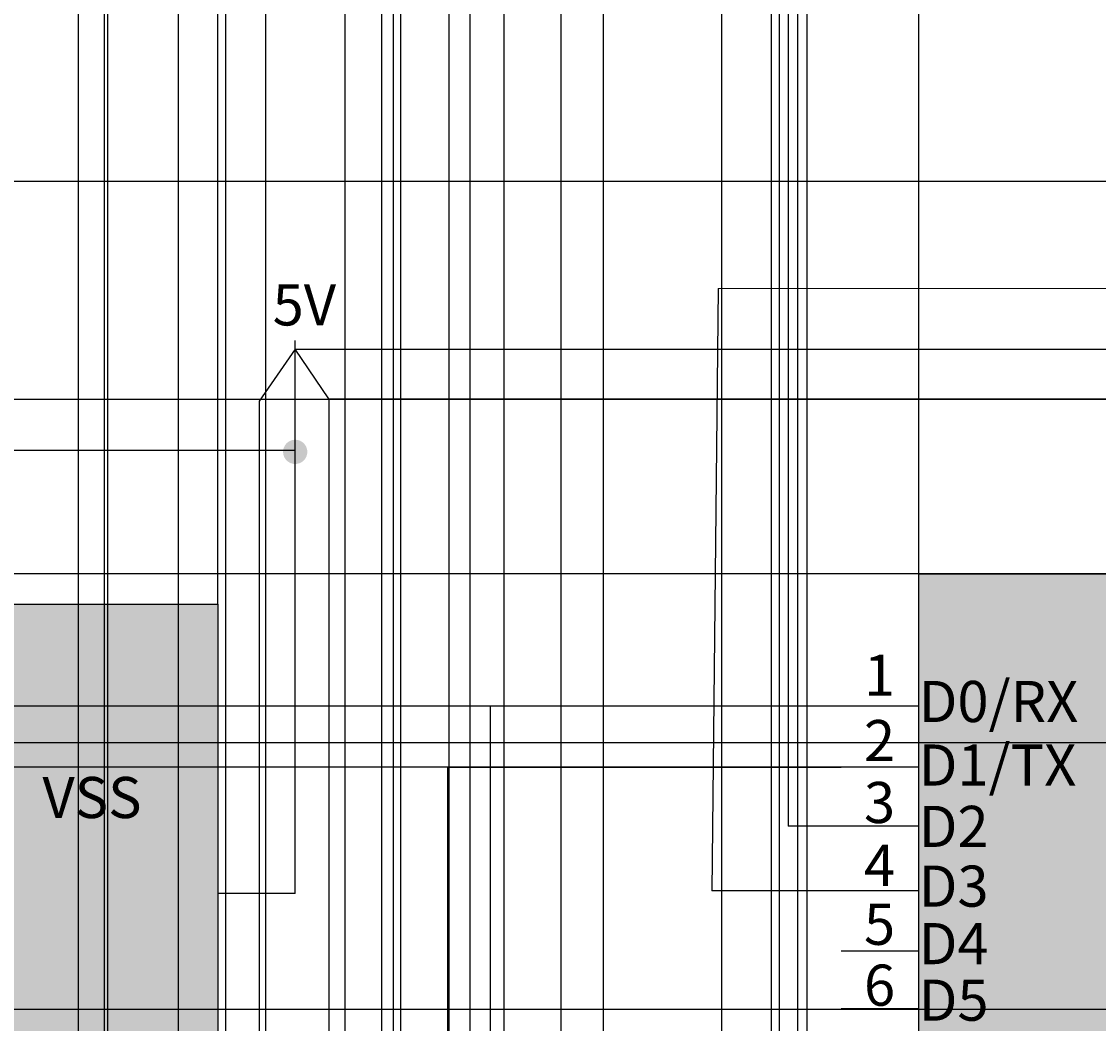
# Model space of a CAD drawing. Units: inches. Extents: x 35362 to 73946, y 43607 to 67532.
# Tile 131 of 134: x 52056 to 57838, y 56772 to 62152. Entities that reach past the tile are written whole.
import ezdxf

# ---------------------------------------------------------------- set-up
doc = ezdxf.new("R2010")
doc.units = ezdxf.units.IN
doc.header["$MEASUREMENT"] = 0
for name, color, linetype, lineweight in [('A-ANNO-DIMS', 2, 'Continuous', 18), ('E-ANNO-TEXT', 5, 'Continuous', 18), ('E-SYMB', 1, 'Continuous', 25), ('E-SYMB-PATT', 1, 'Continuous', 13), ('E-WIRE', 3, 'Continuous', 25)]:
    doc.layers.add(name, color=color, linetype=linetype, lineweight=lineweight)
doc.styles.get("Standard").update_dxf_attribs({"font": 'arial.ttf'})
doc.dimstyles.get("Standard").update_dxf_attribs({"dimtxt": 0.18, "dimasz": 0.18, "dimexe": 0.18, "dimexo": 0.0625, "dimgap": 0.09, "dimtad": 0, "dimtih": 1, "dimtoh": 1, "dimdec": 4, "dimzin": 0, "dimdsep": 46, "dimtxsty": 'Standard', "dimcen": 0.09, "dimadec": 0, "dimazin": 0, "dimtfac": 1, "dimtdec": 4, "dimtofl": 0, "dimtmove": 0, "dimatfit": 3, "dimfxl": 1, "dimtolj": 1, "dimtzin": 0, "dimarcsym": 0})

# ---------------------------------------------------------------- blocks, each defined once
blk = doc.blocks.new('*D9')
at = {"layer": 'A-ANNO-DIMS', "color": 0, "lineweight": -2, "transparency": 16777216}
for p, q in [((56873.6, 59185.2), (56873.6, 67531.7)), ((56873.8, 67531.5), (59056.9, 67531.5)), ((61240.7, 67531.5), (59057.6, 67531.5)), ((61240.9, 59185.2), (61240.9, 67531.7))]:
    blk.add_line(p, q, dxfattribs=at)
at = {"layer": 'A-ANNO-DIMS', "color": 0, "transparency": 16777216}
for points in [[(56873.8, 67531.5), (56873.8, 67531.5), (56873.6, 67531.5)], [(61240.7, 67531.5), (61240.7, 67531.5), (61240.9, 67531.5)]]:
    blk.add_solid(points, dxfattribs=at)
at = {"layer": 'Defpoints', "color": 0, "transparency": 16777216}
for p in [(61240.9, 67531.5), (56873.6, 59185.1), (61240.9, 59185.1)]:
    blk.add_point(p, dxfattribs=at)
at = {"layer": 'A-ANNO-DIMS', "color": 0, "transparency": 16777216, "insert": (59057.3, 67531.5), "char_height": 0.18, "attachment_point": 5}
blk.add_mtext('\\A1;4367', dxfattribs=at)
blk = doc.blocks.new('*D25')
at = {"layer": 'A-ANNO-DIMS', "color": 0, "lineweight": -2, "transparency": 16777216}
for p, q in [((53109.8, 59023.3), (53109.8, 67531.7)), ((53109.9, 67531.5), (54991.2, 67531.5)), ((56873.4, 67531.5), (54992.1, 67531.5)), ((56873.6, 59185.2), (56873.6, 67531.7))]:
    blk.add_line(p, q, dxfattribs=at)
at = {"layer": 'A-ANNO-DIMS', "color": 0, "transparency": 16777216}
for points in [[(53109.9, 67531.5), (53109.9, 67531.5), (53109.8, 67531.5)], [(56873.4, 67531.5), (56873.4, 67531.5), (56873.6, 67531.5)]]:
    blk.add_solid(points, dxfattribs=at)
at = {"layer": 'Defpoints', "color": 0, "transparency": 16777216}
for p in [(56873.6, 67531.5), (56873.6, 59185.1), (53109.8, 59023.3)]:
    blk.add_point(p, dxfattribs=at)
at = {"layer": 'A-ANNO-DIMS', "color": 0, "transparency": 16777216, "insert": (54991.7, 67531.5), "char_height": 0.18, "attachment_point": 5}
blk.add_mtext('\\A1;3763.8', dxfattribs=at)
blk = doc.blocks.new('*D34')
at = {"layer": 'A-ANNO-DIMS', "color": 0, "lineweight": -2, "transparency": 16777216}
for p, q in [((65336, 61293.3), (35361.8, 61293.3)), ((35361.9, 61293.1), (35361.9, 60239.4)), ((35361.9, 59185.3), (35361.9, 60239)), ((61240.8, 59185.1), (35361.8, 59185.1))]:
    blk.add_line(p, q, dxfattribs=at)
at = {"layer": 'A-ANNO-DIMS', "color": 0, "transparency": 16777216}
for points in [[(35361.9, 61293.1), (35362, 61293.1), (35361.9, 61293.3)], [(35361.9, 59185.3), (35362, 59185.3), (35361.9, 59185.1)]]:
    blk.add_solid(points, dxfattribs=at)
at = {"layer": 'Defpoints', "color": 0, "transparency": 16777216}
for p in [(65336, 61293.3), (35361.9, 59185.1), (61240.9, 59185.1)]:
    blk.add_point(p, dxfattribs=at)
at = {"layer": 'A-ANNO-DIMS', "color": 0, "transparency": 16777216, "insert": (35361.9, 60239.2), "char_height": 0.18, "attachment_point": 5}
blk.add_mtext('\\A1;2108.1', dxfattribs=at)
blk = doc.blocks.new('*D36')
at = {"layer": 'A-ANNO-DIMS', "color": 0, "lineweight": -2, "transparency": 16777216}
for p, q in [((68320.8, 60122.3), (35361.8, 60122.3)), ((35361.9, 60122.2), (35361.9, 57247.8)), ((35361.9, 54373.1), (35361.9, 57247.5)), ((68320.8, 54372.9), (35361.8, 54372.9))]:
    blk.add_line(p, q, dxfattribs=at)
at = {"layer": 'A-ANNO-DIMS', "color": 0, "transparency": 16777216}
for points in [[(35361.9, 60122.2), (35362, 60122.2), (35361.9, 60122.3)], [(35361.9, 54373.1), (35362, 54373.1), (35361.9, 54372.9)]]:
    blk.add_solid(points, dxfattribs=at)
at = {"layer": 'Defpoints', "color": 0, "transparency": 16777216}
for p in [(68320.9, 60122.3), (35361.9, 54372.9), (68320.9, 54372.9)]:
    blk.add_point(p, dxfattribs=at)
at = {"layer": 'A-ANNO-DIMS', "color": 0, "transparency": 16777216, "insert": (35361.9, 57247.6), "char_height": 0.18, "attachment_point": 5}
blk.add_mtext('\\A1;5749.4', dxfattribs=at)
blk = doc.blocks.new('*D39')
at = {"layer": 'A-ANNO-DIMS', "color": 0, "lineweight": -2, "transparency": 16777216}
for p, q in [((53793.6, 46128.9), (53793.6, 67531.7)), ((53793.8, 67531.5), (54487.2, 67531.5)), ((55181.5, 67531.5), (54488.1, 67531.5)), ((55181.6, 46128.9), (55181.6, 67531.7))]:
    blk.add_line(p, q, dxfattribs=at)
at = {"layer": 'A-ANNO-DIMS', "color": 0, "transparency": 16777216}
for points in [[(53793.8, 67531.5), (53793.8, 67531.5), (53793.6, 67531.5)], [(55181.5, 67531.5), (55181.5, 67531.5), (55181.6, 67531.5)]]:
    blk.add_solid(points, dxfattribs=at)
at = {"layer": 'Defpoints', "color": 0, "transparency": 16777216}
for p in [(55181.6, 67531.5), (53793.6, 46128.9), (55181.6, 46128.9)]:
    blk.add_point(p, dxfattribs=at)
at = {"layer": 'A-ANNO-DIMS', "color": 0, "transparency": 16777216, "insert": (54487.6, 67531.5), "char_height": 0.18, "attachment_point": 5}
blk.add_mtext('\\A1;1388.0', dxfattribs=at)
blk = doc.blocks.new('*D44')
at = {"layer": 'A-ANNO-DIMS', "color": 0, "lineweight": -2, "transparency": 16777216}
for p, q in [((52517.8, 64828.5), (52517.8, 43606.7)), ((54090.8, 64828.5), (54090.8, 43606.7)), ((52518, 43606.9), (53303.8, 43606.9)), ((54090.6, 43606.9), (53304.7, 43606.9))]:
    blk.add_line(p, q, dxfattribs=at)
at = {"layer": 'A-ANNO-DIMS', "color": 0, "transparency": 16777216}
for points in [[(52518, 43606.9), (52518, 43606.8), (52517.8, 43606.9)], [(54090.6, 43606.9), (54090.6, 43606.8), (54090.8, 43606.9)]]:
    blk.add_solid(points, dxfattribs=at)
at = {"layer": 'Defpoints', "color": 0, "transparency": 16777216}
for p in [(52517.8, 64828.6), (54090.8, 64828.6), (54090.8, 43606.9)]:
    blk.add_point(p, dxfattribs=at)
at = {"layer": 'A-ANNO-DIMS', "color": 0, "transparency": 16777216, "insert": (53304.3, 43606.9), "char_height": 0.18, "attachment_point": 5}
blk.add_mtext('\\A1;1573.0', dxfattribs=at)
blk = doc.blocks.new('*D47')
at = {"layer": 'A-ANNO-DIMS', "color": 0, "lineweight": -2, "transparency": 16777216}
for p, q in [((50339.6, 58280), (73945.8, 58280)), ((73945.6, 58279.8), (73945.6, 57564.2)), ((73945.6, 56848.2), (73945.6, 57563.8)), ((50339.6, 56848), (73945.8, 56848))]:
    blk.add_line(p, q, dxfattribs=at)
at = {"layer": 'A-ANNO-DIMS', "color": 0, "transparency": 16777216}
for points in [[(73945.6, 58279.8), (73945.7, 58279.8), (73945.6, 58280)], [(73945.6, 56848.2), (73945.7, 56848.2), (73945.6, 56848)]]:
    blk.add_solid(points, dxfattribs=at)
at = {"layer": 'Defpoints', "color": 0, "transparency": 16777216}
for p in [(50339.5, 58280), (50339.5, 56848), (73945.6, 56848)]:
    blk.add_point(p, dxfattribs=at)
at = {"layer": 'A-ANNO-DIMS', "color": 0, "transparency": 16777216, "insert": (73945.6, 57564), "char_height": 0.18, "attachment_point": 5}
blk.add_mtext('\\A1;1432.0', dxfattribs=at)
blk = doc.blocks.new('*D48')
at = {"layer": 'A-ANNO-DIMS', "color": 0, "lineweight": -2, "transparency": 16777216}
for p, q in [((56457.2, 58474.9), (35361.8, 58474.9)), ((35361.9, 58474.7), (35361.9, 58311.1)), ((35361.9, 58147.1), (35361.9, 58310.7)), ((56457.2, 58147), (35361.8, 58147))]:
    blk.add_line(p, q, dxfattribs=at)
at = {"layer": 'A-ANNO-DIMS', "color": 0, "transparency": 16777216}
for points in [[(35361.9, 58474.7), (35362, 58474.7), (35361.9, 58474.9)], [(35361.9, 58147.1), (35362, 58147.1), (35361.9, 58147)]]:
    blk.add_solid(points, dxfattribs=at)
at = {"layer": 'Defpoints', "color": 0, "transparency": 16777216}
for p in [(56457.3, 58474.9), (35361.9, 58147), (56457.3, 58147)]:
    blk.add_point(p, dxfattribs=at)
at = {"layer": 'A-ANNO-DIMS', "color": 0, "transparency": 16777216, "insert": (35361.9, 58310.9), "char_height": 0.18, "attachment_point": 5}
blk.add_mtext('\\A1;327.9', dxfattribs=at)
blk = doc.blocks.new('*D51')
at = {"layer": 'A-ANNO-DIMS', "color": 0, "lineweight": -2, "transparency": 16777216}
for p, q in [((56873.6, 59185.2), (56873.6, 67531.7)), ((56873.8, 67531.5), (57886, 67531.5)), ((58899.2, 67531.5), (57887, 67531.5)), ((58899.4, 59601.5), (58899.4, 67531.7))]:
    blk.add_line(p, q, dxfattribs=at)
at = {"layer": 'A-ANNO-DIMS', "color": 0, "transparency": 16777216}
for points in [[(56873.8, 67531.5), (56873.8, 67531.5), (56873.6, 67531.5)], [(58899.2, 67531.5), (58899.2, 67531.5), (58899.4, 67531.5)]]:
    blk.add_solid(points, dxfattribs=at)
at = {"layer": 'Defpoints', "color": 0, "transparency": 16777216}
for p in [(58899.4, 67531.5), (58899.4, 59601.5), (56873.6, 59185.1)]:
    blk.add_point(p, dxfattribs=at)
at = {"layer": 'A-ANNO-DIMS', "color": 0, "transparency": 16777216, "insert": (57886.5, 67531.5), "char_height": 0.18, "attachment_point": 5}
blk.add_mtext('\\A1;2025.8', dxfattribs=at)
blk = doc.blocks.new('*D77')
at = {"layer": 'A-ANNO-DIMS', "color": 0, "lineweight": -2, "transparency": 16777216}
for p, q in [((53793.6, 46128.9), (53793.6, 67531.7)), ((53793.8, 67531.5), (53922.8, 67531.5)), ((54052.7, 67531.5), (53923.7, 67531.5)), ((54052.9, 46555.4), (54052.9, 67531.7))]:
    blk.add_line(p, q, dxfattribs=at)
at = {"layer": 'A-ANNO-DIMS', "color": 0, "transparency": 16777216}
for points in [[(53793.8, 67531.5), (53793.8, 67531.5), (53793.6, 67531.5)], [(54052.7, 67531.5), (54052.7, 67531.5), (54052.9, 67531.5)]]:
    blk.add_solid(points, dxfattribs=at)
at = {"layer": 'Defpoints', "color": 0, "transparency": 16777216}
for p in [(54052.9, 67531.5), (54052.9, 46555.3), (53793.6, 46128.9)]:
    blk.add_point(p, dxfattribs=at)
at = {"layer": 'A-ANNO-DIMS', "color": 0, "transparency": 16777216, "insert": (53923.3, 67531.5), "char_height": 0.18, "attachment_point": 5}
blk.add_mtext('\\A1;259.26', dxfattribs=at)
blk = doc.blocks.new('*D78')
at = {"layer": 'A-ANNO-DIMS', "color": 0, "lineweight": -2, "transparency": 16777216}
for p, q in [((54052.9, 46555.4), (54052.9, 67531.7)), ((54053.1, 67531.5), (54202.6, 67531.5)), ((54352.9, 67531.5), (54203.4, 67531.5)), ((54353.1, 46555.4), (54353.1, 67531.7))]:
    blk.add_line(p, q, dxfattribs=at)
at = {"layer": 'A-ANNO-DIMS', "color": 0, "transparency": 16777216}
for points in [[(54053.1, 67531.5), (54053.1, 67531.5), (54052.9, 67531.5)], [(54352.9, 67531.5), (54352.9, 67531.5), (54353.1, 67531.5)]]:
    blk.add_solid(points, dxfattribs=at)
at = {"layer": 'Defpoints', "color": 0, "transparency": 16777216}
for p in [(54353.1, 67531.5), (54052.9, 46555.3), (54353.1, 46555.3)]:
    blk.add_point(p, dxfattribs=at)
at = {"layer": 'A-ANNO-DIMS', "color": 0, "transparency": 16777216, "insert": (54203, 67531.5), "char_height": 0.18, "attachment_point": 5}
blk.add_mtext('\\A1;300.2', dxfattribs=at)
blk = doc.blocks.new('*D79')
at = {"layer": 'A-ANNO-DIMS', "color": 0, "lineweight": -2, "transparency": 16777216}
for p, q in [((54353.1, 46555.4), (54353.1, 67531.7)), ((54353.3, 67531.5), (54500.2, 67531.5)), ((54648, 67531.5), (54501, 67531.5)), ((54648.2, 46555.4), (54648.2, 67531.7))]:
    blk.add_line(p, q, dxfattribs=at)
at = {"layer": 'A-ANNO-DIMS', "color": 0, "transparency": 16777216}
for points in [[(54353.3, 67531.5), (54353.3, 67531.5), (54353.1, 67531.5)], [(54648, 67531.5), (54648, 67531.5), (54648.2, 67531.5)]]:
    blk.add_solid(points, dxfattribs=at)
at = {"layer": 'Defpoints', "color": 0, "transparency": 16777216}
for p in [(54648.2, 67531.5), (54353.1, 46555.3), (54648.2, 46555.3)]:
    blk.add_point(p, dxfattribs=at)
at = {"layer": 'A-ANNO-DIMS', "color": 0, "transparency": 16777216, "insert": (54500.6, 67531.5), "char_height": 0.18, "attachment_point": 5}
blk.add_mtext('\\A1;295.1', dxfattribs=at)
blk = doc.blocks.new('*D80')
at = {"layer": 'A-ANNO-DIMS', "color": 0, "lineweight": -2, "transparency": 16777216}
for p, q in [((54648.2, 46555.4), (54648.2, 67531.7)), ((54648.4, 67531.5), (54800.3, 67531.5)), ((54953.3, 67531.5), (54801.3, 67531.5)), ((54953.4, 46555.4), (54953.4, 67531.7))]:
    blk.add_line(p, q, dxfattribs=at)
at = {"layer": 'A-ANNO-DIMS', "color": 0, "transparency": 16777216}
for points in [[(54648.4, 67531.5), (54648.4, 67531.5), (54648.2, 67531.5)], [(54953.3, 67531.5), (54953.3, 67531.5), (54953.4, 67531.5)]]:
    blk.add_solid(points, dxfattribs=at)
at = {"layer": 'Defpoints', "color": 0, "transparency": 16777216}
for p in [(54953.4, 67531.5), (54648.2, 46555.3), (54953.4, 46555.3)]:
    blk.add_point(p, dxfattribs=at)
at = {"layer": 'A-ANNO-DIMS', "color": 0, "transparency": 16777216, "insert": (54800.8, 67531.5), "char_height": 0.18, "attachment_point": 5}
blk.add_mtext('\\A1;305.27', dxfattribs=at)
blk = doc.blocks.new('*D82')
at = {"layer": 'A-ANNO-DIMS', "color": 0, "lineweight": -2, "transparency": 16777216}
for p, q in [((54464.4, 49314.7), (54464.4, 67531.7)), ((54464.6, 67531.5), (55139.4, 67531.5)), ((55815.1, 67531.5), (55140.3, 67531.5)), ((55815.3, 49110.2), (55815.3, 67531.7))]:
    blk.add_line(p, q, dxfattribs=at)
at = {"layer": 'A-ANNO-DIMS', "color": 0, "transparency": 16777216}
for points in [[(54464.6, 67531.5), (54464.6, 67531.5), (54464.4, 67531.5)], [(55815.1, 67531.5), (55815.1, 67531.5), (55815.3, 67531.5)]]:
    blk.add_solid(points, dxfattribs=at)
at = {"layer": 'Defpoints', "color": 0, "transparency": 16777216}
for p in [(55815.3, 67531.5), (54464.4, 49314.7), (55815.3, 49110.1)]:
    blk.add_point(p, dxfattribs=at)
at = {"layer": 'A-ANNO-DIMS', "color": 0, "transparency": 16777216, "insert": (55139.9, 67531.5), "char_height": 0.18, "attachment_point": 5}
blk.add_mtext('\\A1;1350.9', dxfattribs=at)
blk = doc.blocks.new('*D88')
at = {"layer": 'A-ANNO-DIMS', "color": 0, "lineweight": -2, "transparency": 16777216}
for p, q in [((52362.6, 48318.3), (52362.6, 67531.7)), ((52362.7, 67531.5), (52432.1, 67531.5)), ((52502.2, 67531.5), (52432.8, 67531.5)), ((52502.4, 48318.3), (52502.4, 67531.7))]:
    blk.add_line(p, q, dxfattribs=at)
at = {"layer": 'A-ANNO-DIMS', "color": 0, "transparency": 16777216}
for points in [[(52362.7, 67531.5), (52362.7, 67531.5), (52362.6, 67531.5)], [(52502.2, 67531.5), (52502.2, 67531.5), (52502.4, 67531.5)]]:
    blk.add_solid(points, dxfattribs=at)
at = {"layer": 'Defpoints', "color": 0, "transparency": 16777216}
for p in [(52502.4, 67531.5), (52362.6, 48318.3), (52502.4, 48318.3)]:
    blk.add_point(p, dxfattribs=at)
at = {"layer": 'A-ANNO-DIMS', "color": 0, "transparency": 16777216, "insert": (52432.5, 67531.5), "char_height": 0.18, "attachment_point": 5}
blk.add_mtext('\\A1;139.8', dxfattribs=at)
blk = doc.blocks.new('*D96')
at = {"layer": 'A-ANNO-DIMS', "color": 0, "lineweight": -2, "transparency": 16777216}
for p, q in [((53366.8, 64997.6), (53366.8, 43606.7)), ((53988.6, 64997.6), (53988.6, 43606.7)), ((53366.9, 43606.9), (53677.3, 43606.9)), ((53988.4, 43606.9), (53678.1, 43606.9))]:
    blk.add_line(p, q, dxfattribs=at)
at = {"layer": 'A-ANNO-DIMS', "color": 0, "transparency": 16777216}
for points in [[(53366.9, 43606.9), (53366.9, 43606.8), (53366.8, 43606.9)], [(53988.4, 43606.9), (53988.4, 43606.8), (53988.6, 43606.9)]]:
    blk.add_solid(points, dxfattribs=at)
at = {"layer": 'Defpoints', "color": 0, "transparency": 16777216}
for p in [(53366.8, 64997.7), (53988.6, 64997.7), (53988.6, 43606.9)]:
    blk.add_point(p, dxfattribs=at)
at = {"layer": 'A-ANNO-DIMS', "color": 0, "transparency": 16777216, "insert": (53677.7, 43606.9), "char_height": 0.18, "attachment_point": 5}
blk.add_mtext('\\A1;621.8', dxfattribs=at)
blk = doc.blocks.new('*D99')
at = {"layer": 'A-ANNO-DIMS', "color": 0, "lineweight": -2, "transparency": 16777216}
for p, q in [((52897.5, 65291.5), (52897.5, 43606.7)), ((52517.8, 64828.5), (52517.8, 43606.7)), ((52518, 43606.9), (52707.2, 43606.9)), ((52897.3, 43606.9), (52708, 43606.9))]:
    blk.add_line(p, q, dxfattribs=at)
at = {"layer": 'A-ANNO-DIMS', "color": 0, "transparency": 16777216}
for points in [[(52518, 43606.9), (52518, 43606.8), (52517.8, 43606.9)], [(52897.3, 43606.9), (52897.3, 43606.8), (52897.5, 43606.9)]]:
    blk.add_solid(points, dxfattribs=at)
at = {"layer": 'Defpoints', "color": 0, "transparency": 16777216}
for p in [(52897.5, 65291.6), (52517.8, 64828.6), (52897.5, 43606.9)]:
    blk.add_point(p, dxfattribs=at)
at = {"layer": 'A-ANNO-DIMS', "color": 0, "transparency": 16777216, "insert": (52707.6, 43606.9), "char_height": 0.18, "attachment_point": 5}
blk.add_mtext('\\A1;379.7', dxfattribs=at)
blk = doc.blocks.new('*D100')
at = {"layer": 'A-ANNO-DIMS', "color": 0, "lineweight": -2, "transparency": 16777216}
for p, q in [((52897.5, 65291.5), (52897.5, 43606.7)), ((53150.7, 64926.1), (53150.7, 43606.7)), ((52897.7, 43606.9), (53023.7, 43606.9)), ((53150.5, 43606.9), (53024.5, 43606.9))]:
    blk.add_line(p, q, dxfattribs=at)
at = {"layer": 'A-ANNO-DIMS', "color": 0, "transparency": 16777216}
for points in [[(52897.7, 43606.9), (52897.7, 43606.8), (52897.5, 43606.9)], [(53150.5, 43606.9), (53150.5, 43606.8), (53150.7, 43606.9)]]:
    blk.add_solid(points, dxfattribs=at)
at = {"layer": 'Defpoints', "color": 0, "transparency": 16777216}
for p in [(52897.5, 65291.6), (53150.7, 64926.1), (53150.7, 43606.9)]:
    blk.add_point(p, dxfattribs=at)
at = {"layer": 'A-ANNO-DIMS', "color": 0, "transparency": 16777216, "insert": (53024.1, 43606.9), "char_height": 0.18, "attachment_point": 5}
blk.add_mtext('\\A1;253.2', dxfattribs=at)
blk = doc.blocks.new('*D102')
at = {"layer": 'A-ANNO-DIMS', "color": 0, "lineweight": -2, "transparency": 16777216}
for p, q in [((56080.5, 63694.7), (56080.5, 43606.7)), ((56272.5, 63696.8), (56272.5, 43606.7)), ((56080.7, 43606.9), (56176, 43606.9)), ((56272.3, 43606.9), (56176.9, 43606.9))]:
    blk.add_line(p, q, dxfattribs=at)
at = {"layer": 'A-ANNO-DIMS', "color": 0, "transparency": 16777216}
for points in [[(56080.7, 43606.9), (56080.7, 43606.8), (56080.5, 43606.9)], [(56272.3, 43606.9), (56272.3, 43606.8), (56272.5, 43606.9)]]:
    blk.add_solid(points, dxfattribs=at)
at = {"layer": 'Defpoints', "color": 0, "transparency": 16777216}
for p in [(56080.5, 63694.8), (56272.5, 63696.9), (56272.5, 43606.9)]:
    blk.add_point(p, dxfattribs=at)
at = {"layer": 'A-ANNO-DIMS', "color": 0, "transparency": 16777216, "insert": (56176.5, 43606.9), "char_height": 0.18, "attachment_point": 5}
blk.add_mtext('\\A1;191.98', dxfattribs=at)
blk = doc.blocks.new('*D104')
at = {"layer": 'A-ANNO-DIMS', "color": 0, "lineweight": -2, "transparency": 16777216}
for p, q in [((56123.2, 63318.1), (56123.2, 43606.7)), ((56223, 63318.1), (56223, 43606.7)), ((56123.4, 43606.9), (56172.7, 43606.9)), ((56222.8, 43606.9), (56173.5, 43606.9))]:
    blk.add_line(p, q, dxfattribs=at)
at = {"layer": 'A-ANNO-DIMS', "color": 0, "transparency": 16777216}
for points in [[(56123.4, 43606.9), (56123.4, 43606.8), (56123.2, 43606.9)], [(56222.8, 43606.9), (56222.8, 43606.8), (56223, 43606.9)]]:
    blk.add_solid(points, dxfattribs=at)
at = {"layer": 'Defpoints', "color": 0, "transparency": 16777216}
for p in [(56123.2, 63318.1), (56223, 63318.1), (56223, 43606.9)]:
    blk.add_point(p, dxfattribs=at)
at = {"layer": 'A-ANNO-DIMS', "color": 0, "transparency": 16777216, "insert": (56173.1, 43606.9), "char_height": 0.18, "attachment_point": 5}
blk.add_mtext('\\A1;99.74', dxfattribs=at)
blk = doc.blocks.new('*D112')
at = {"layer": 'A-ANNO-DIMS', "color": 0, "lineweight": -2, "transparency": 16777216}
for p, q in [((53332.8, 60113.4), (53332.8, 43606.7)), ((53705.4, 60126.2), (53705.4, 43606.7)), ((53332.9, 43606.9), (53518.7, 43606.9)), ((53705.2, 43606.9), (53519.5, 43606.9))]:
    blk.add_line(p, q, dxfattribs=at)
at = {"layer": 'A-ANNO-DIMS', "color": 0, "transparency": 16777216}
for points in [[(53332.9, 43606.9), (53332.9, 43606.8), (53332.8, 43606.9)], [(53705.2, 43606.9), (53705.2, 43606.8), (53705.4, 43606.9)]]:
    blk.add_solid(points, dxfattribs=at)
at = {"layer": 'Defpoints', "color": 0, "transparency": 16777216}
for p in [(53332.8, 60113.5), (53705.4, 60126.3), (53705.4, 43606.9)]:
    blk.add_point(p, dxfattribs=at)
at = {"layer": 'A-ANNO-DIMS', "color": 0, "transparency": 16777216, "insert": (53519.1, 43606.9), "char_height": 0.18, "attachment_point": 5}
blk.add_mtext('\\A1;372.6', dxfattribs=at)
blk = doc.blocks.new('*D113')
at = {"layer": 'A-ANNO-DIMS', "color": 0, "lineweight": -2, "transparency": 16777216}
for p, q in [((53526.1, 60391.7), (73945.8, 60391.7)), ((73945.6, 60391.5), (73945.6, 60259.2)), ((73945.6, 60126.5), (73945.6, 60258.8)), ((53705.4, 60126.3), (73945.8, 60126.3))]:
    blk.add_line(p, q, dxfattribs=at)
at = {"layer": 'A-ANNO-DIMS', "color": 0, "transparency": 16777216}
for points in [[(73945.6, 60391.5), (73945.7, 60391.5), (73945.6, 60391.7)], [(73945.6, 60126.5), (73945.7, 60126.5), (73945.6, 60126.3)]]:
    blk.add_solid(points, dxfattribs=at)
at = {"layer": 'Defpoints', "color": 0, "transparency": 16777216}
for p in [(53526.1, 60391.7), (73945.6, 60391.7), (53705.4, 60126.3)]:
    blk.add_point(p, dxfattribs=at)
at = {"layer": 'A-ANNO-DIMS', "color": 0, "transparency": 16777216, "insert": (73945.6, 60259), "char_height": 0.18, "attachment_point": 5}
blk.add_mtext('\\A1;265.4', dxfattribs=at)

msp = doc.modelspace()

# ---------------------------------------------------------------- hatches: boundary and pattern name
at = {"layer": 'E-SYMB-PATT'}
h = msp.add_hatch(color=256, dxfattribs=at)
h.dxf.hatch_style = 1
h.paths.add_polyline_path([(53525.64, 59906.061, 0.41421356), (53460.435, 59840.856, 0.41421356), (53525.64, 59775.651)])
h.paths.add_polyline_path([(53525.64, 59906.061), (53525.64, 59775.651, 0.41421356), (53590.844, 59840.856, 0.41421356)])
h = msp.add_hatch(color=256, dxfattribs=at)
h.dxf.hatch_style = 1
h.paths.add_polyline_path([(56873.602, 59185.144), (56873.602, 53351.529), (61240.907, 53351.529), (61240.907, 59185.144)])
h = msp.add_hatch(color=256, dxfattribs=at)
h.dxf.hatch_style = 1
h.paths.add_polyline_path([(53109.76, 56028.836), (53109.76, 59023.276), (47978.665, 59023.276), (47978.665, 56028.836)])

# ---------------------------------------------------------------- linework, layer by layer
at = {"layer": 'E-SYMB'}
for p, q in [((53526.072, 60391.719), (53332.762, 60113.464)), ((53526.072, 59850.077), (53526.072, 60391.719)), ((53705.36, 60126.3), (53526.072, 60391.719)), ((56873.602, 58474.868), (56457.29, 58474.868)), ((56873.602, 58146.959), (56457.29, 58146.959)), ((56873.602, 57830.141), (56457.29, 57830.141)), ((56873.602, 57483.492), (56457.29, 57483.492)), ((53526.072, 57468.896), (53109.76, 57468.896)), ((56873.602, 57159.65), (56457.29, 57159.65)), ((56873.602, 56849.491), (56457.29, 56849.491))]:
    msp.add_line(p, q, dxfattribs=at)
for points in [[(56873.602, 59185.144), (61240.907, 59185.144), (61240.907, 53351.529), (56873.602, 53351.529)], [(47978.665, 59023.276), (53109.76, 59023.276), (53109.76, 56028.836), (47978.665, 56028.836)]]:
    msp.add_lwpolyline(points, close=True, dxfattribs=at)
at = {"layer": 'E-WIRE'}
for p, q in [((56172.082, 63247.066), (56172.082, 57830.141)), ((55796.172, 60718.228), (55762.055, 57483.492)), ((55796.172, 60718.228), (61077.865, 60722.339)), ((53526.072, 57468.896), (53526.072, 60439.178)), ((51612.51, 59850.077), (53526.072, 59850.077)), ((56457.29, 58474.868), (54572.84, 58474.868)), ((54572.84, 58474.868), (54572.84, 52004.266)), ((54344.773, 53911.892), (54344.773, 58146.959)), ((54344.773, 58146.959), (56457.29, 58146.959)), ((56457.29, 57830.141), (56172.082, 57830.141)), ((56457.29, 57483.492), (55762.055, 57483.492))]:
    msp.add_line(p, q, dxfattribs=at)

# ---------------------------------------------------------------- texts
at = {"layer": 'E-ANNO-TEXT'}
for s, p in [('5V', (53404.472, 60519.588)), ('1', (56579.272, 58531.071)), ('D0/RX', (56873.602, 58390.038)), ('2', (56579.272, 58180.002)), ('D1/TX', (56873.602, 58048.675)), ('VSS', (52168.54, 57874.469)), ('3', (56579.272, 57847.684)), ('D2', (56873.602, 57719.22)), ('4', (56579.272, 57510.186)), ('D3', (56873.602, 57398.578)), ('5', (56579.272, 57193.79)), ('D4', (56873.602, 57089.937)), ('6', (56579.272, 56866.73)), ('D5', (56873.602, 56786.254))]:
    msp.add_text(s, height=220.866, dxfattribs=at).set_placement(p)

# ---------------------------------------------------------------- dimensions: what is measured, and where the dimension line sits
at = {"layer": 'A-ANNO-DIMS'}
for base, p1, p2, override, picture, middle in [((52502.363, 67531.512), (52362.557, 48318.269), (52502.363, 48318.269), {"dimdec": 1, "dimlfac": 1, "dimrnd": 0, "dimzin": 0, "dimdsep": 46, "dimlunit": 2}, '*D88', (52432.46, 67531.512)), ((56873.602, 67531.512), (53109.76, 59023.276), (56873.602, 59185.144), {"dimdec": 1, "dimlfac": 1, "dimrnd": 0, "dimzin": 0, "dimdsep": 46, "dimlunit": 2}, '*D25', (54991.681, 67531.512)), ((55181.634, 67531.512), (53793.638, 46128.878), (55181.634, 46128.878), {"dimdec": 1, "dimlfac": 1, "dimrnd": 0, "dimzin": 0, "dimdsep": 46, "dimlunit": 2}, '*D39', (54487.636, 67531.512)), ((54052.899, 67531.512), (53793.638, 46128.878), (54052.899, 46555.293), {"dimdec": 2, "dimlfac": 1, "dimrnd": 0, "dimzin": 0, "dimdsep": 46, "dimlunit": 2}, '*D77', (53923.269, 67531.512)), ((54353.08, 67531.512), (54052.899, 46555.293), (54353.08, 46555.293), {"dimdec": 1, "dimlfac": 1, "dimrnd": 0, "dimzin": 0, "dimdsep": 46, "dimlunit": 2}, '*D78', (54202.99, 67531.512)), ((54648.173, 67531.512), (54353.08, 46555.293), (54648.173, 46555.293), {"dimdec": 1, "dimlfac": 1, "dimrnd": 0, "dimzin": 0, "dimdsep": 46, "dimlunit": 2}, '*D79', (54500.627, 67531.512)), ((55815.319, 67531.512), (54464.399, 49314.669), (55815.319, 49110.104), {"dimdec": 1, "dimlfac": 1, "dimrnd": 0, "dimzin": 0, "dimdsep": 46, "dimlunit": 2}, '*D82', (55139.859, 67531.512)), ((54953.441, 67531.512), (54648.173, 46555.293), (54953.441, 46555.293), {"dimdec": 2, "dimlfac": 1, "dimrnd": 0, "dimzin": 0, "dimdsep": 46, "dimlunit": 2}, '*D80', (54800.807, 67531.512)), ((61240.907, 67531.512), (56873.602, 59185.144), (61240.907, 59185.144), {"dimdec": 0, "dimlfac": 1, "dimrnd": 0, "dimzin": 0, "dimdsep": 46, "dimlunit": 2}, '*D9', (59057.255, 67531.512)), ((58899.392, 67531.512), (56873.602, 59185.144), (58899.392, 59601.456), {"dimdec": 1, "dimlfac": 1, "dimrnd": 0, "dimzin": 0, "dimdsep": 46, "dimlunit": 2}, '*D51', (57886.497, 67531.512)), ((52897.48, 43606.859), (52517.798, 64828.556), (52897.48, 65291.589), {"dimdec": 1, "dimlfac": 1, "dimrnd": 0, "dimzin": 0, "dimdsep": 46, "dimlunit": 2}, '*D99', (52707.639, 43606.859)), ((53150.662, 43606.859), (52897.48, 65291.589), (53150.662, 64926.138), {"dimdec": 1, "dimlfac": 1, "dimrnd": 0, "dimzin": 0, "dimdsep": 46, "dimlunit": 2}, '*D100', (53024.071, 43606.859)), ((53988.6156, 43606.859), (53366.7657, 64997.6827), (53988.6156, 64997.6827), {"dimdec": 1, "dimlfac": 1, "dimrnd": 0, "dimzin": 0, "dimdsep": 46, "dimlunit": 2}, '*D96', (53677.6907, 43606.859)), ((54090.768, 43606.859), (52517.798, 64828.556), (54090.768, 64828.556), {"dimdec": 1, "dimlfac": 1, "dimrnd": 0, "dimzin": 0, "dimdsep": 46, "dimlunit": 2}, '*D44', (53304.283, 43606.859)), ((56272.469, 43606.859), (56080.488, 63694.755), (56272.469, 63696.867), {"dimdec": 2, "dimlfac": 1, "dimrnd": 0, "dimzin": 0, "dimdsep": 46, "dimlunit": 2}, '*D102', (56176.479, 43606.859)), ((56222.953, 43606.859), (56123.213, 63318.132), (56222.953, 63318.132), {"dimdec": 2, "dimlfac": 1, "dimrnd": 0, "dimzin": 0, "dimdsep": 46, "dimlunit": 2}, '*D104', (56173.083, 43606.859)), ((53705.36, 43606.859), (53332.762, 60113.464), (53705.36, 60126.3), {"dimdec": 1, "dimlfac": 1, "dimrnd": 0, "dimzin": 0, "dimdsep": 46, "dimlunit": 2}, '*D112', (53519.061, 43606.859))]:
    dim = msp.add_linear_dim(base=base, p1=p1, p2=p2, dimstyle='Standard', override=override, dxfattribs=at)
    dim.commit()
    dim.dimension.update_dxf_attribs({"geometry": picture, "text_midpoint": middle})
for base, p1, p2, picture, middle in [((35361.949, 59185.144), (65336.016, 61293.286), (61240.907, 59185.144), '*D34', (35361.949, 60239.215)), ((73945.646, 60391.719), (53705.36, 60126.3), (53526.072, 60391.719), '*D113', (73945.646, 60259.01)), ((35361.949, 54372.948), (68320.871, 60122.346), (68320.871, 54372.948), '*D36', (35361.949, 57247.647)), ((35361.949, 58146.959), (56457.29, 58474.868), (56457.29, 58146.959), '*D48', (35361.949, 58310.914)), ((73945.646, 56847.99), (50339.524, 58279.988), (50339.524, 56847.99), '*D47', (73945.646, 57563.989))]:
    dim = msp.add_linear_dim(base=base, p1=p1, p2=p2, angle=90, dimstyle='Standard', override={"dimdec": 1, "dimlfac": 1, "dimrnd": 0, "dimzin": 0, "dimdsep": 46, "dimlunit": 2}, dxfattribs=at)
    dim.commit()
    dim.dimension.update_dxf_attribs({"geometry": picture, "text_midpoint": middle})

doc.saveas('drawing.dxf')
